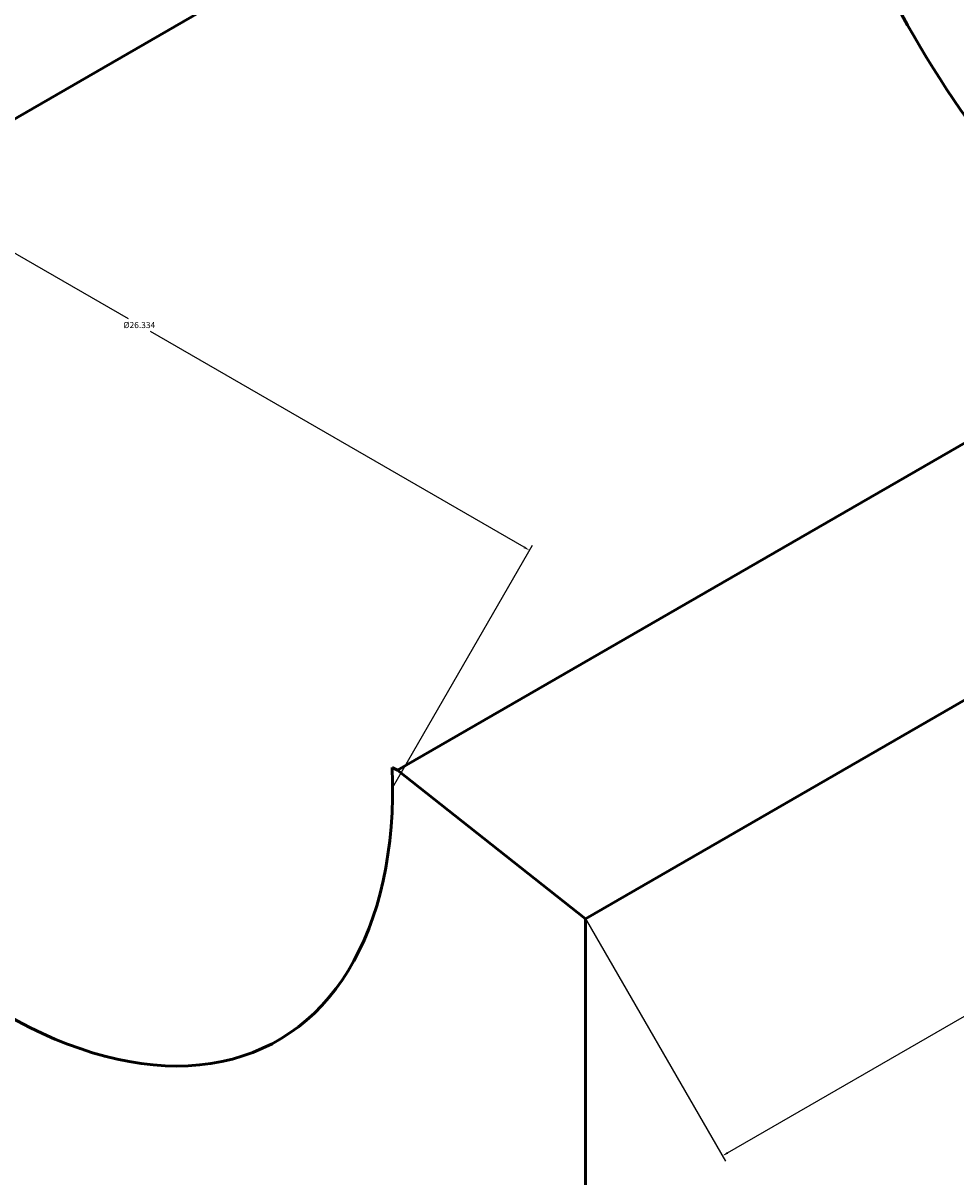
# Model space of a CAD drawing. Units: millimetres. Extents: x 2919 to 3075, y 2801 to 2951.
# Tile 6 of 14: x 2979 to 3006, y 2876 to 2910. Entities that reach past the tile are written whole.
import ezdxf

# ---------------------------------------------------------------- set-up
doc = ezdxf.new("R2010")
doc.units = ezdxf.units.MM
doc.layers.add('M-DIMS', color=2, linetype='Continuous', lineweight=18)
doc.layers.add('M-OUTL', color=7, linetype='Continuous', lineweight=50)
doc.styles.get("Standard").update_dxf_attribs({"font": 'arial.ttf'})
doc.dimstyles.get("Standard").update_dxf_attribs({"dimtxt": 0.18, "dimasz": 0.18, "dimexe": 0.18, "dimexo": 0.0625, "dimgap": 0.09, "dimtad": 0, "dimtih": 1, "dimtoh": 1, "dimdec": 4, "dimzin": 0, "dimdsep": 46, "dimtxsty": 'Standard', "dimcen": 0.09, "dimadec": 0, "dimazin": 0, "dimtfac": 1, "dimtdec": 4, "dimtofl": 0, "dimtmove": 0, "dimatfit": 3, "dimfxl": 1, "dimtolj": 1, "dimtzin": 0, "dimarcsym": 0})

# ---------------------------------------------------------------- blocks, each defined once
blk = doc.blocks.new('*D1')
at = {"layer": 'Defpoints', "color": 0, "transparency": 16777216}
for p in [(2987.323, 2944.203), (3074.337, 2944.203), (3010.912, 2808.893)]:
    blk.add_point(p, dxfattribs=at)
at = {"layer": 'M-DIMS', "color": 0, "lineweight": -2, "transparency": 16777216}
for p, q in [((2987.386, 2944.203), (3074.517, 2944.203)), ((3074.337, 2944.023), (3074.337, 2876.73)), ((3074.337, 2809.073), (3074.337, 2876.366)), ((3010.974, 2808.893), (3074.517, 2808.893))]:
    blk.add_line(p, q, dxfattribs=at)
at = {"layer": 'M-DIMS', "color": 0, "transparency": 16777216}
for points in [[(3074.307, 2944.023), (3074.367, 2944.023), (3074.337, 2944.203)], [(3074.307, 2809.073), (3074.367, 2809.073), (3074.337, 2808.893)]]:
    blk.add_solid(points, dxfattribs=at)
at = {"layer": 'M-DIMS', "color": 0, "transparency": 16777216, "insert": (3074.337, 2876.548), "char_height": 0.18, "attachment_point": 5}
blk.add_mtext('\\A1;135.3', dxfattribs=at)
blk = doc.blocks.new('*D12')
at = {"layer": 'Defpoints', "color": 0, "transparency": 16777216}
for p in [(3031.696, 2904.893), (2995.323, 2883.893), (2999.323, 2876.965)]:
    blk.add_point(p, dxfattribs=at)
at = {"layer": 'M-DIMS', "color": 0, "lineweight": -2, "transparency": 16777216}
for p, q in [((3031.727, 2904.839), (3035.786, 2897.809)), ((3035.54, 2897.875), (3017.731, 2887.593)), ((2999.479, 2877.055), (3017.288, 2887.337)), ((2995.354, 2883.839), (2999.413, 2876.809))]:
    blk.add_line(p, q, dxfattribs=at)
at = {"layer": 'M-DIMS', "color": 0, "transparency": 16777216}
for points in [[(3035.525, 2897.901), (3035.555, 2897.849), (3035.696, 2897.965)], [(2999.464, 2877.081), (2999.494, 2877.029), (2999.323, 2876.965)]]:
    blk.add_solid(points, dxfattribs=at)
at = {"layer": 'M-DIMS', "color": 0, "transparency": 16777216, "insert": (3017.51, 2887.465), "char_height": 0.18, "attachment_point": 5}
blk.add_mtext('\\A1;42', dxfattribs=at)
blk = doc.blocks.new('*D17')
at = {"layer": 'Defpoints', "color": 0, "transparency": 16777216}
for p in [(2966.884, 2900.897), (2993.691, 2894.658), (2989.691, 2887.729)]:
    blk.add_point(p, dxfattribs=at)
at = {"layer": 'M-DIMS', "color": 0, "lineweight": -2, "transparency": 16777216}
for p, q in [((2966.915, 2900.951), (2970.974, 2907.981)), ((2971.04, 2907.735), (2981.964, 2901.428)), ((2993.535, 2894.748), (2982.611, 2901.054)), ((2989.722, 2887.783), (2993.781, 2894.813))]:
    blk.add_line(p, q, dxfattribs=at)
at = {"layer": 'M-DIMS', "color": 0, "transparency": 16777216}
for points in [[(2971.055, 2907.761), (2971.025, 2907.709), (2970.884, 2907.825)], [(2993.55, 2894.774), (2993.52, 2894.722), (2993.691, 2894.658)]]:
    blk.add_solid(points, dxfattribs=at)
at = {"layer": 'M-DIMS', "color": 0, "transparency": 16777216, "insert": (2982.287, 2901.241), "char_height": 0.18, "attachment_point": 5}
blk.add_mtext('\\A1;%%c26.334', dxfattribs=at)
blk = doc.blocks.new('*D18')
at = {"layer": 'Defpoints', "color": 0, "transparency": 16777216}
for p in [(3001.241, 2922.061), (3030.348, 2914.493), (3026.348, 2907.565)]:
    blk.add_point(p, dxfattribs=at)
at = {"layer": 'M-DIMS', "color": 0, "lineweight": -2, "transparency": 16777216}
for p, q in [((3001.272, 2922.115), (3005.331, 2929.145)), ((3005.397, 2928.899), (3017.471, 2921.928)), ((3030.192, 2914.583), (3018.118, 2921.554)), ((3026.379, 2907.619), (3030.438, 2914.649))]:
    blk.add_line(p, q, dxfattribs=at)
at = {"layer": 'M-DIMS', "color": 0, "transparency": 16777216}
for points in [[(3005.412, 2928.925), (3005.382, 2928.873), (3005.241, 2928.989)], [(3030.207, 2914.609), (3030.177, 2914.557), (3030.348, 2914.493)]]:
    blk.add_solid(points, dxfattribs=at)
at = {"layer": 'M-DIMS', "color": 0, "transparency": 16777216, "insert": (3017.794, 2921.741), "char_height": 0.18, "attachment_point": 5}
blk.add_mtext('\\A1;%%c28.99', dxfattribs=at)

msp = doc.modelspace()

# ---------------------------------------------------------------- linework, layer by layer
at = {"layer": 'M-OUTL'}
for p, q in [((2966.7443, 2900.3932), (3001.3853, 2920.3932)), ((2989.8305, 2888.2326), (3026.2035, 2909.2326)), ((2995.3232, 2883.8932), (3021.3039, 2898.8932)), ((2989.6796, 2888.3121), (2989.8305, 2888.2326)), ((2995.3232, 2883.8932), (2989.8305, 2888.2326)), ((2995.3232, 2855.8932), (2995.3232, 2883.8932))]:
    msp.add_line(p, q, dxfattribs=at)
for centre, major_axis, start_param, end_param in [((3013.7944, 2914.8129), (8.8766, -15.3748), 4.0414742, 5.3833038), ((2978.2874, 2894.3129), (8.0632, -13.966), 3.9585863, 7.1123769)]:
    msp.add_ellipse(centre, major_axis=major_axis, ratio=0.5773503, start_param=start_param, end_param=end_param, dxfattribs=at)

# ---------------------------------------------------------------- dimensions: what is measured, and where the dimension line sits
at = {"layer": 'M-DIMS'}
for base, p1, p2, angle, override, picture, middle in [((3074.3372, 2944.2026), (3010.9116, 2808.8932), (2987.3232, 2944.2026), 90, {"dimdec": 1, "dimlfac": 1, "dimrnd": 0, "dimzin": 0, "dimdsep": 46, "dimlunit": 2}, '*D1', (3074.3372, 2876.5479)), ((2999.3232, 2876.965), (3031.6962, 2904.8932), (2995.3232, 2883.8932), 210, {"dimdec": 0, "dimlfac": 1, "dimrnd": 0, "dimzin": 0, "dimdsep": 46, "dimlunit": 2}, '*D12', (3017.5097, 2887.465))]:
    dim = msp.add_linear_dim(base=base, p1=p1, p2=p2, angle=angle, dimstyle='Standard', override=override, dxfattribs=at)
    dim.commit()
    dim.dimension.update_dxf_attribs({"geometry": picture, "text_midpoint": middle})
for base, p1, p2, override, picture, middle in [((3030.3479, 2914.4934), (3001.241, 2922.0607), (3026.3479, 2907.5652), {"dimdec": 2, "dimlfac": 1, "dimrnd": 0, "dimzin": 0, "dimdsep": 46, "dimlunit": 2}, '*D18', (3017.7944, 2921.7411)), ((2993.69055, 2894.65752), (2966.88424, 2900.89655), (2989.69055, 2887.72932), {"dimdec": 3, "dimlfac": 1, "dimrnd": 0, "dimzin": 0, "dimdsep": 46, "dimlunit": 2}, '*D17', (2982.2874, 2901.24114))]:
    dim = msp.add_linear_dim(base=base, p1=p1, p2=p2, angle=330, text='%%c<>', dimstyle='Standard', override=override, dxfattribs=at)
    dim.commit()
    dim.dimension.update_dxf_attribs({"geometry": picture, "text_midpoint": middle})

doc.saveas('drawing.dxf')
